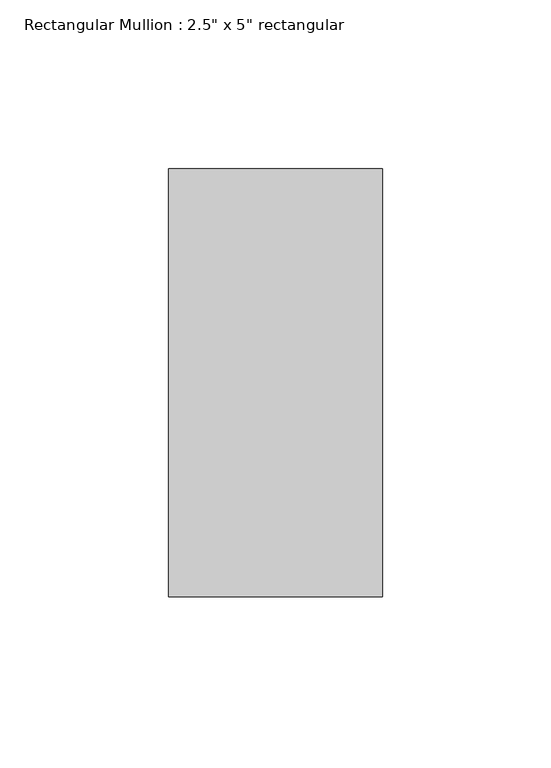
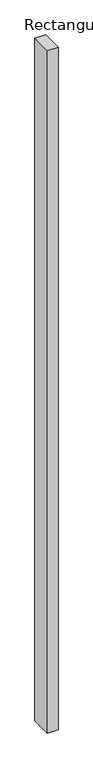
"""IFC4 building model written with IfcOpenShell, lengths in millimetres: member geometry."""

from ifc_helpers import new_model, si_unit, frame, origin, place, context, project, spatial, polyline, outline, extrude, source, transform, mapped, element, save


def member_9e61c091(model_context):
    return source(origin(), model_context, "Body", "SweptSolid", [
        extrude(outline(polyline([(31.75, 63.5), (31.75, -63.5), (-31.75, -63.5), (-31.75, 63.5), (31.75, 63.5)])), frame((0.0, 0.0, -4267.2), z_axis=(0.0, 0.0, 1.0), x_axis=(1.0, 0.0, 0.0)), (0.0, 0.0, 1.0), 4267.2),
    ])


if __name__ == "__main__":
    model = new_model("IFC4")
    model_context = context("Model", 3, world=origin())
    ifc_project = project(units=[si_unit("LENGTHUNIT", "METRE", prefix="MILLI")], contexts=[model_context])
    site = spatial("IfcSite", under=ifc_project)
    building = spatial("IfcBuilding", under=site)
    placement = place(None, origin())
    member_shape = member_9e61c091(model_context)
    element("IfcMember", 1, ObjectType="Rectangular Mullion : 2.5\" x 5\" rectangular", at=placement, inside=building, context=model_context, shape_type="MappedRepresentation", body=[
        mapped(member_shape, transform((0.0, 0.0, 0.0), x_axis=(1.0, 0.0, 0.0), y_axis=(0.0, 1.0, 0.0), z_axis=(0.0, 0.0, 1.0))),
    ])
    save(model, "model.ifc")

# Revit data of these elements
# Type "Rectangular Mullion : 2.5\" x 5\" rectangular"
#   built-in parameter 1007304 = 0.416667 (stored number, unit not read)
#   built-in parameter 1007301 = 0.104167 (stored number, unit not read)
#   built-in parameter 1007300 = 0.104167 (stored number, unit not read)
# Element 1 (IfcMember, "Rectangular Mullion : 2.5\" x 5\" rectangular")
#   Materials on its faces: "Iron, Ductile"
# Materials
#   "Iron, Ductile": class "Metal", colour RGB 0 0 0, transparency 0, Description = "Ductile cast iron", Cost = 0
